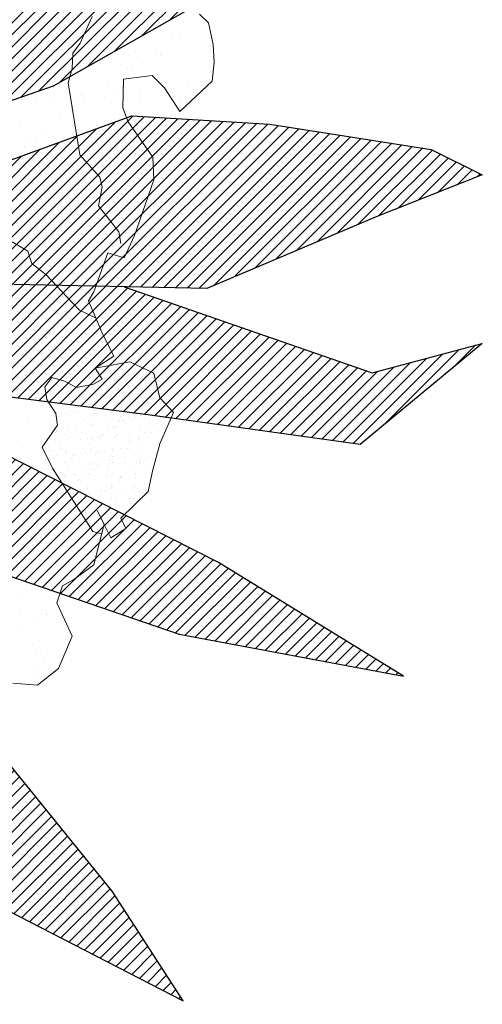
# Model space of a CAD drawing. Units: inches. Extents: x 1986 to 21484, y -1816 to 2016.
# Tile 71 of 85: x 3679.11 to 3687.55, y 1870.8 to 1888.79. Entities that reach past the tile are written whole.
import ezdxf

# ---------------------------------------------------------------- set-up
doc = ezdxf.new("R2010")
doc.units = ezdxf.units.IN
doc.layers.add('L-PLNT', color=84, linetype='Continuous', lineweight=13)
doc.layers.add('vfolhas', color=114, linetype='Continuous', lineweight=5)
for name, color, linetype in [('vfolha', 72, 'Continuous'), ('vfolha2', 110, 'Continuous'), ('vfolhas2', 102, 'Continuous')]:
    doc.layers.add(name, color=color, linetype=linetype)
pattern_1 = [(45, (-2446.5133113, 50.986076), (-0.004419417382, 0.004419417382), [])]

# ---------------------------------------------------------------- blocks, each defined once
blk = doc.blocks.new('arbusto_PB_verde_grande')
at = {"layer": 'vfolha2'}
h = blk.add_hatch(dxfattribs=at)
h.set_pattern_fill('ANSI31', color=256, scale=0.05, style=0)
h.set_pattern_definition(pattern_1)
h.paths.add_polyline_path([(0.02944, 0.35651), (0.00028, 0.09048), (0.02625, -0.03934), (0.047, 0.06233), (0.06189, 0.09731), (0.09372, 0.26573), (0.09955, 0.43473), (0.08789, 0.61313), (0.0645, 0.72266), (0.04988, 0.6851), (0.0236, 0.51294)])
h.paths.add_polyline_path([(0.30106, 0.43789), (0.14225, 0.24871), (0.26685, 0.30022)])
h.paths.add_polyline_path([(0.37995, 0.22817), (0.23697, 0.15193), (0.18428, 0.09364), (0.11122, 0.04358), (0.02625, -0.03934), (0.28061, 0.04667), (0.36829, 0.07798), (0.46756, 0.11239), (0.61068, 0.19376), (0.71585, 0.27823), (0.55813, 0.25948)])
h.paths.add_polyline_path([(0.56101, -0.29441), (0.72752, -0.32573), (0.59024, -0.2412), (0.42962, -0.15982), (0.02625, -0.03934), (0.14922, -0.14107), (0.18838, -0.16604), (0.41501, -0.24435)])
h.paths.add_polyline_path([(-0.27429, -0.44776), (-0.30352, -0.72628), (-0.23923, -0.64175), (-0.15457, -0.45716), (0.02625, -0.03934), (-0.16328, -0.25376)])
h.paths.add_polyline_path([(-0.51963, -0.24744), (-0.67736, -0.32573), (-0.59558, -0.35072), (-0.40574, -0.32882), (-0.21007, -0.20995), (0.02625, -0.03934), (-0.14874, -0.06595), (-0.31518, -0.09101), (-0.41452, -0.15048)])
h.paths.add_polyline_path([(-0.52546, 0.25007), (-0.70947, 0.24698), (-0.51963, 0.1093), (-0.32979, 0.02167), (-0.07567, -0.0128), (-0.04234, -0.02148), (-0.35024, 0.1312)])
at = {"layer": 'vfolhas'}
h = blk.add_hatch(dxfattribs=at)
h.set_pattern_fill('ANSI31', color=256, scale=0.05, style=0)
h.set_pattern_definition(pattern_1)
h.paths.add_polyline_path([(-0.07279, 0.50669), (-0.18085, 0.65063), (-0.2334, 0.67253), (-0.20712, 0.53176), (-0.10785, 0.25007), (0.02625, -0.03934), (0.00028, 0.09048), (0.00816, 0.16241), (-0.04939, 0.29079)])
h.paths.add_polyline_path([(0.09902, 0.41929), (0.09372, 0.26573), (0.07906, 0.18814), (0.15506, 0.36901), (0.26606, 0.5505), (0.28356, 0.63504), (0.2485, 0.68819), (0.25145, 0.63504), (0.20178, 0.54426)])
h.paths.add_polyline_path([(0.12295, 0.24073), (0.047, 0.06233), (0.02625, -0.03934), (0.11122, 0.04358), (0.18428, 0.09364), (0.27478, 0.19376), (0.3215, 0.25323), (0.44129, 0.38467), (0.47634, 0.57866), (0.41789, 0.45347), (0.28939, 0.30954)])
h.paths.add_polyline_path([(0.58145, -0.03779), (0.70707, 0.01536), (0.78591, 0.04667), (0.74796, 0.06549), (0.62818, 0.08423), (0.52595, 0.09048), (0.39745, 0.04358), (0.02625, -0.03934), (0.25728, -0.03154), (0.43834, -0.0347)])
h.paths.add_polyline_path([(0.52022, -0.03647), (0.43834, -0.0347), (0.25728, -0.03154), (0.02625, -0.03934), (0.17964, -0.08515), (0.53768, -0.13167), (0.69541, -0.15357), (0.78591, -0.07852), (0.70413, -0.10042)])
h.paths.add_polyline_path([(0.27189, -0.21929), (0.14922, -0.14107), (0.02625, -0.03934), (0.15794, -0.31007), (0.29522, -0.42585), (0.41789, -0.49157), (0.56396, -0.56669), (0.5114, -0.48532), (0.39456, -0.34139)])
h.paths.add_polyline_path([(-0.05818, -0.47591), (-0.02312, -0.61984), (0.047, -0.80134), (0.08494, -0.59794), (0.07911, -0.4071), (0.03527, -0.25376), (0.02625, -0.03934), (-0.03773, -0.26001)])
h.paths.add_polyline_path([(-0.24218, 0.14054), (-0.11073, 0.06858), (0.02625, -0.03934), (-0.04235, 0.10871), (-0.21007, 0.23757), (-0.36485, 0.33145), (-0.47874, 0.40341), (-0.54303, 0.46288), (-0.49041, 0.33145), (-0.39408, 0.22192)])
at = {"layer": 'vfolha'}
for p, q in [((0.52022, -0.03647), (0.70413, -0.10042)), ((0.78591, -0.07852), (0.69541, -0.15357)), ((0.70413, -0.10042), (0.78591, -0.07852)), ((0.53768, -0.13167), (0.17964, -0.08515)), ((0.69541, -0.15357), (0.53768, -0.13167)), ((0.5114, -0.48532), (0.39456, -0.34139)), ((0.56396, -0.56669), (0.5114, -0.48532)), ((0.41789, -0.49157), (0.56396, -0.56669))]:
    blk.add_line(p, q, dxfattribs=at)
at = {"layer": 'vfolha2'}
for p, q in [((0.61068, 0.19376), (0.46756, 0.11239)), ((0.59024, -0.2412), (0.42962, -0.15982)), ((0.72752, -0.32573), (0.59024, -0.2412)), ((0.41501, -0.24435), (0.56101, -0.29441)), ((0.56101, -0.29441), (0.72752, -0.32573))]:
    blk.add_line(p, q, dxfattribs=at)
at = {"layer": 'vfolhas2'}
for p, q in [((0.46756, 0.11239), (0.36829, 0.07798)), ((0.39745, 0.04358), (0.52595, 0.09048)), ((0.52595, 0.09048), (0.62818, 0.08423)), ((0.62818, 0.08423), (0.74796, 0.06549)), ((0.74796, 0.06549), (0.78591, 0.04667)), ((0.78591, 0.04667), (0.70707, 0.01536)), ((0.70707, 0.01536), (0.58145, -0.03779)), ((0.58145, -0.03779), (0.43834, -0.0347))]:
    blk.add_line(p, q, dxfattribs=at)
blk = doc.blocks.new('PLANT-SHRUB')
for p, q in [((2160.298, 1902.236), (2160.882, 1902.496)), ((2160.882, 1902.496), (2161.373, 1902.455)), ((2161.373, 1902.455), (2161.676, 1902.121)), ((2160.089, 1901.6), (2160.298, 1902.236)), ((2160.978, 1902.218), (2160.978, 1902.218)), ((2161.178, 1902.255), (2161.178, 1902.255)), ((2161.252, 1902.322), (2161.252, 1902.322)), ((2160.81, 1902.111), (2160.81, 1902.111)), ((2160.78, 1901.89), (2160.78, 1901.89)), ((2160.942, 1901.982), (2160.942, 1901.982)), ((2159.805, 1901.685), (2159.805, 1901.685)), ((2158.177, 1901.273), (2158.24, 1901.471)), ((2158.24, 1901.471), (2158.553, 1901.409)), ((2158.474, 1901.143), (2159.119, 1901.558)), ((2159.119, 1901.558), (2159.568, 1901.506)), ((2159.119, 1901.558), (2159.119, 1901.558)), ((2159.568, 1901.506), (2159.797, 1901.443)), ((2159.797, 1901.443), (2160.089, 1901.6)), ((2160.018, 1901.606), (2160.018, 1901.606)), ((2160.348, 1901.614), (2160.348, 1901.614)), ((2160.359, 1901.504), (2160.359, 1901.504)), ((2160.377, 1901.625), (2160.377, 1901.625)), ((2160.433, 1901.571), (2160.433, 1901.571)), ((2160.556, 1901.586), (2160.556, 1901.586)), ((2160.881, 1901.543), (2160.881, 1901.543)), ((2157.478, 1901.263), (2158.177, 1901.273)), ((2158.553, 1901.409), (2158.396, 1900.877)), ((2158.497, 1901.332), (2158.497, 1901.332)), ((2157.165, 1901.044), (2157.478, 1901.263)), ((2157.596, 1901.148), (2157.596, 1901.148)), ((2157.679, 1901.137), (2157.679, 1901.137)), ((2157.753, 1901.169), (2157.753, 1901.169)), ((2157.795, 1901.116), (2157.795, 1901.116)), ((2157.809, 1901.12), (2157.809, 1901.12)), ((2157.862, 1901.187), (2157.862, 1901.187)), ((2157.862, 1901.159), (2157.862, 1901.159)), ((2157.998, 1901.115), (2157.998, 1901.115)), ((2158.026, 1901.091), (2158.026, 1901.091)), ((2158.166, 1901.222), (2158.166, 1901.222)), ((2158.293, 1901.115), (2158.293, 1901.115)), ((2158.294, 1901.171), (2158.294, 1901.171)), ((2158.338, 1901.104), (2158.338, 1901.104)), ((2158.36, 1901.158), (2158.36, 1901.158)), ((2158.393, 1901.174), (2158.393, 1901.174)), ((2158.396, 1900.877), (2158.474, 1901.143)), ((2158.412, 1901.172), (2158.412, 1901.172)), ((2158.423, 1901.201), (2158.423, 1901.201)), ((2158.46, 1899.75), (2158.716, 1901.103)), ((2158.716, 1901.103), (2158.627, 1901.241)), ((2158.791, 1901.264), (2158.791, 1901.264)), ((2159.242, 1901.112), (2159.242, 1901.112)), ((2159.411, 1901.22), (2159.411, 1901.22)), ((2159.87, 1901.225), (2159.87, 1901.225)), ((2159.961, 1901.139), (2159.961, 1901.139)), ((2160.487, 1901.11), (2160.487, 1901.11)), ((2160.655, 1901.218), (2160.655, 1901.218)), ((2156.726, 1900.772), (2157.165, 1901.044)), ((2156.98, 1900.915), (2156.98, 1900.915)), ((2157.285, 1900.982), (2157.285, 1900.982)), ((2157.478, 1900.914), (2157.478, 1900.914)), ((2157.585, 1901.014), (2157.585, 1901.014)), ((2157.614, 1901.041), (2157.614, 1901.041)), ((2157.659, 1901.027), (2157.659, 1901.027)), ((2157.828, 1900.91), (2157.828, 1900.91)), ((2157.976, 1900.913), (2157.976, 1900.913)), ((2158.078, 1901.022), (2158.078, 1901.022)), ((2158.11, 1901.08), (2158.11, 1901.08)), ((2158.234, 1901.028), (2158.234, 1901.028)), ((2158.24, 1901.063), (2158.24, 1901.063)), ((2158.457, 1901.035), (2158.457, 1901.035)), ((2158.474, 1900.912), (2158.474, 1900.912)), ((2158.487, 1901.024), (2158.487, 1901.024)), ((2158.54, 1901.024), (2158.54, 1901.024)), ((2158.67, 1901.007), (2158.67, 1901.007)), ((2156.152, 1900.522), (2156.726, 1900.772)), ((2156.737, 1900.76), (2156.737, 1900.76)), ((2156.808, 1900.732), (2156.808, 1900.732)), ((2157.018, 1900.81), (2157.018, 1900.81)), ((2157.025, 1900.882), (2157.025, 1900.882)), ((2157.102, 1900.799), (2157.102, 1900.799)), ((2157.204, 1900.902), (2157.204, 1900.902)), ((2157.217, 1900.734), (2157.217, 1900.734)), ((2157.231, 1900.782), (2157.231, 1900.782)), ((2157.235, 1900.759), (2157.235, 1900.759)), ((2157.287, 1900.741), (2157.287, 1900.741)), ((2157.426, 1900.868), (2157.426, 1900.868)), ((2157.443, 1900.877), (2157.443, 1900.877)), ((2157.449, 1900.753), (2157.449, 1900.753)), ((2157.532, 1900.742), (2157.532, 1900.742)), ((2157.733, 1900.758), (2157.733, 1900.758)), ((2157.852, 1900.879), (2157.852, 1900.879)), ((2157.941, 1900.74), (2157.941, 1900.74)), ((2158.036, 1900.883), (2158.036, 1900.883)), ((2158.065, 1900.874), (2158.065, 1900.874)), ((2158.095, 1900.901), (2158.095, 1900.901)), ((2158.231, 1900.757), (2158.231, 1900.757)), ((2158.284, 1900.863), (2158.284, 1900.863)), ((2158.284, 1900.863), (2158.284, 1900.863)), ((2158.361, 1900.84), (2158.361, 1900.84)), ((2158.546, 1900.734), (2158.546, 1900.734)), ((2158.575, 1900.761), (2158.575, 1900.761)), ((2158.904, 1900.769), (2158.904, 1900.769)), ((2159.112, 1900.741), (2159.112, 1900.741)), ((2159.33, 1900.85), (2159.33, 1900.85)), ((2159.54, 1900.753), (2159.54, 1900.753)), ((2159.614, 1900.821), (2159.614, 1900.821)), ((2156.449, 1900.554), (2156.449, 1900.554)), ((2156.478, 1900.581), (2156.478, 1900.581)), ((2156.583, 1900.59), (2156.583, 1900.59)), ((2156.617, 1900.709), (2156.617, 1900.709)), ((2156.67, 1900.717), (2156.67, 1900.717)), ((2157.014, 1900.574), (2157.014, 1900.574)), ((2157.098, 1900.568), (2157.098, 1900.568)), ((2157.168, 1900.716), (2157.168, 1900.716)), ((2157.206, 1900.61), (2157.206, 1900.61)), ((2157.257, 1900.714), (2157.257, 1900.714)), ((2157.433, 1900.569), (2157.433, 1900.569)), ((2157.649, 1900.719), (2157.649, 1900.719)), ((2157.662, 1900.725), (2157.662, 1900.725)), ((2157.666, 1900.715), (2157.666, 1900.715)), ((2157.738, 1900.574), (2157.738, 1900.574)), ((2157.767, 1900.601), (2157.767, 1900.601)), ((2157.842, 1900.571), (2157.842, 1900.571)), ((2157.879, 1900.697), (2157.879, 1900.697)), ((2157.906, 1900.728), (2157.906, 1900.728)), ((2157.962, 1900.686), (2157.962, 1900.686)), ((2158.068, 1900.714), (2158.068, 1900.714)), ((2158.092, 1900.669), (2158.092, 1900.669)), ((2158.163, 1900.714), (2158.163, 1900.714)), ((2158.274, 1900.555), (2158.274, 1900.555)), ((2158.309, 1900.64), (2158.309, 1900.64)), ((2158.387, 1900.588), (2158.387, 1900.588)), ((2158.392, 1900.629), (2158.392, 1900.629)), ((2158.45, 1900.608), (2158.45, 1900.608)), ((2158.477, 1900.715), (2158.477, 1900.715)), ((2158.522, 1900.612), (2158.522, 1900.612)), ((2159.437, 1900.699), (2159.437, 1900.699)), ((2159.695, 1900.606), (2159.695, 1900.606)), ((2159.979, 1900.627), (2159.979, 1900.627)), ((2156.152, 1900.157), (2156.152, 1900.522)), ((2156.38, 1900.43), (2156.38, 1900.43)), ((2156.441, 1900.472), (2156.441, 1900.472)), ((2156.524, 1900.461), (2156.524, 1900.461)), ((2156.654, 1900.444), (2156.654, 1900.444)), ((2156.697, 1900.502), (2156.697, 1900.502)), ((2156.798, 1900.424), (2156.798, 1900.424)), ((2156.851, 1900.514), (2156.851, 1900.514)), ((2156.871, 1900.416), (2156.871, 1900.416)), ((2156.929, 1900.414), (2156.929, 1900.414)), ((2156.954, 1900.405), (2156.954, 1900.405)), ((2156.959, 1900.441), (2156.959, 1900.441)), ((2157.084, 1900.388), (2157.084, 1900.388)), ((2157.207, 1900.426), (2157.207, 1900.426)), ((2157.349, 1900.513), (2157.349, 1900.513)), ((2157.579, 1900.428), (2157.579, 1900.428)), ((2157.593, 1900.421), (2157.593, 1900.421)), ((2157.639, 1900.411), (2157.639, 1900.411)), ((2157.743, 1900.489), (2157.743, 1900.489)), ((2157.847, 1900.513), (2157.847, 1900.513)), ((2158.057, 1900.405), (2158.057, 1900.405)), ((2158.218, 1900.433), (2158.218, 1900.433)), ((2158.248, 1900.46), (2158.248, 1900.46)), ((2158.344, 1900.512), (2158.344, 1900.512)), ((2158.466, 1900.407), (2158.466, 1900.407)), ((2158.766, 1900.494), (2158.766, 1900.494)), ((2159.142, 1900.389), (2159.142, 1900.389)), ((2159.845, 1900.455), (2159.845, 1900.455)), ((2156.541, 1900.317), (2156.541, 1900.317)), ((2156.573, 1900.282), (2156.573, 1900.282)), ((2156.599, 1900.224), (2156.599, 1900.224)), ((2156.608, 1900.36), (2156.608, 1900.36)), ((2156.77, 1900.268), (2156.77, 1900.268)), ((2157.004, 1900.266), (2157.004, 1900.266)), ((2157.039, 1900.316), (2157.039, 1900.316)), ((2157.106, 1900.359), (2157.106, 1900.359)), ((2157.301, 1900.359), (2157.301, 1900.359)), ((2157.384, 1900.348), (2157.384, 1900.348)), ((2157.41, 1900.273), (2157.41, 1900.273)), ((2157.423, 1900.261), (2157.423, 1900.261)), ((2157.44, 1900.3), (2157.44, 1900.3)), ((2157.514, 1900.331), (2157.514, 1900.331)), ((2157.519, 1900.353), (2157.519, 1900.353)), ((2157.537, 1900.315), (2157.537, 1900.315)), ((2157.604, 1900.358), (2157.604, 1900.358)), ((2157.732, 1900.302), (2157.732, 1900.302)), ((2157.815, 1900.291), (2157.815, 1900.291)), ((2157.832, 1900.263), (2157.832, 1900.263)), ((2157.843, 1900.221), (2157.843, 1900.221)), ((2157.945, 1900.274), (2157.945, 1900.274)), ((2158.034, 1900.314), (2158.034, 1900.314)), ((2158.059, 1900.288), (2158.059, 1900.288)), ((2158.102, 1900.357), (2158.102, 1900.357)), ((2158.162, 1900.246), (2158.162, 1900.246)), ((2158.245, 1900.235), (2158.245, 1900.235)), ((2158.264, 1900.247), (2158.264, 1900.247)), ((2158.375, 1900.218), (2158.375, 1900.218)), ((2158.532, 1900.313), (2158.532, 1900.313)), ((2159.088, 1900.219), (2159.088, 1900.219)), ((2155.923, 1899.751), (2156.152, 1900.157)), ((2156.157, 1900.127), (2156.157, 1900.127)), ((2156.224, 1900.115), (2156.224, 1900.115)), ((2156.293, 1900.078), (2156.293, 1900.078)), ((2156.37, 1900.122), (2156.37, 1900.122)), ((2156.376, 1900.067), (2156.376, 1900.067)), ((2156.384, 1900.066), (2156.384, 1900.066)), ((2156.43, 1900.116), (2156.43, 1900.116)), ((2156.506, 1900.05), (2156.506, 1900.05)), ((2156.592, 1900.038), (2156.592, 1900.038)), ((2156.602, 1900.114), (2156.602, 1900.114)), ((2156.631, 1900.141), (2156.631, 1900.141)), ((2156.722, 1900.114), (2156.722, 1900.114)), ((2156.723, 1900.021), (2156.723, 1900.021)), ((2156.788, 1900.116), (2156.788, 1900.116)), ((2156.807, 1900.01), (2156.807, 1900.01)), ((2157.179, 1900.132), (2157.179, 1900.132)), ((2157.197, 1900.118), (2157.197, 1900.118)), ((2157.22, 1900.113), (2157.22, 1900.113)), ((2157.251, 1900.128), (2157.251, 1900.128)), ((2157.629, 1900.103), (2157.629, 1900.103)), ((2157.675, 1900.114), (2157.675, 1900.114)), ((2157.718, 1900.112), (2157.718, 1900.112)), ((2157.891, 1900.133), (2157.891, 1900.133)), ((2157.92, 1900.16), (2157.92, 1900.16)), ((2158.047, 1900.097), (2158.047, 1900.097)), ((2158.215, 1900.111), (2158.215, 1900.111)), ((2158.259, 1900.093), (2158.259, 1900.093)), ((2158.401, 1900.02), (2158.401, 1900.02)), ((2158.456, 1900.099), (2158.456, 1900.099)), ((2158.794, 1900.07), (2158.794, 1900.07)), ((2158.919, 1900.112), (2158.919, 1900.112)), ((2159.305, 1900.08), (2159.305, 1900.08)), ((2156.154, 1899.972), (2156.154, 1899.972)), ((2156.304, 1899.84), (2156.304, 1899.84)), ((2156.412, 1899.916), (2156.412, 1899.916)), ((2156.443, 1899.968), (2156.443, 1899.968)), ((2156.479, 1899.959), (2156.479, 1899.959)), ((2156.563, 1899.974), (2156.563, 1899.974)), ((2156.91, 1899.916), (2156.91, 1899.916)), ((2156.916, 1899.996), (2156.916, 1899.996)), ((2156.937, 1899.993), (2156.937, 1899.993)), ((2156.977, 1899.958), (2156.977, 1899.958)), ((2156.994, 1899.958), (2156.994, 1899.958)), ((2157.082, 1899.973), (2157.082, 1899.973)), ((2157.112, 1900), (2157.112, 1900)), ((2157.121, 1899.989), (2157.121, 1899.989)), ((2157.154, 1899.964), (2157.154, 1899.964)), ((2157.237, 1899.953), (2157.237, 1899.953)), ((2157.367, 1899.936), (2157.367, 1899.936)), ((2157.407, 1899.915), (2157.407, 1899.915)), ((2157.413, 1899.953), (2157.413, 1899.953)), ((2157.459, 1899.924), (2157.459, 1899.924)), ((2157.475, 1899.958), (2157.475, 1899.958)), ((2157.563, 1899.833), (2157.563, 1899.833)), ((2157.584, 1899.908), (2157.584, 1899.908)), ((2157.592, 1899.86), (2157.592, 1899.86)), ((2157.667, 1899.897), (2157.667, 1899.897)), ((2157.667, 1899.897), (2157.667, 1899.897)), ((2157.732, 1899.987), (2157.732, 1899.987)), ((2157.797, 1899.88), (2157.797, 1899.88)), ((2157.822, 1899.955), (2157.822, 1899.955)), ((2157.905, 1899.914), (2157.905, 1899.914)), ((2157.973, 1899.957), (2157.973, 1899.957)), ((2157.992, 1899.854), (2157.992, 1899.854)), ((2158.014, 1899.851), (2158.014, 1899.851)), ((2158.098, 1899.84), (2158.098, 1899.84)), ((2158.212, 1899.847), (2158.212, 1899.847)), ((2158.254, 1899.939), (2158.254, 1899.939)), ((2158.371, 1899.993), (2158.371, 1899.993)), ((2158.403, 1899.913), (2158.403, 1899.913)), ((2158.471, 1899.956), (2158.471, 1899.956)), ((2158.721, 1900.003), (2158.721, 1900.003)), ((2156.102, 1899.305), (2155.923, 1899.751)), ((2156.095, 1899.715), (2156.095, 1899.715)), ((2156.115, 1899.667), (2156.115, 1899.667)), ((2156.143, 1899.664), (2156.143, 1899.664)), ((2156.146, 1899.683), (2156.146, 1899.683)), ((2156.229, 1899.672), (2156.229, 1899.672)), ((2156.274, 1899.813), (2156.274, 1899.813)), ((2156.359, 1899.655), (2156.359, 1899.655)), ((2156.36, 1899.814), (2156.36, 1899.814)), ((2156.552, 1899.666), (2156.552, 1899.666)), ((2156.593, 1899.714), (2156.593, 1899.714)), ((2156.672, 1899.732), (2156.672, 1899.732)), ((2156.755, 1899.673), (2156.755, 1899.673)), ((2156.774, 1899.67), (2156.774, 1899.67)), ((2156.778, 1899.808), (2156.778, 1899.808)), ((2156.784, 1899.7), (2156.784, 1899.7)), ((2156.923, 1899.827), (2156.923, 1899.827)), ((2157.091, 1899.713), (2157.091, 1899.713)), ((2157.187, 1899.81), (2157.187, 1899.81)), ((2157.404, 1899.687), (2157.404, 1899.687)), ((2157.588, 1899.712), (2157.588, 1899.712)), ((2157.619, 1899.795), (2157.619, 1899.795)), ((2157.718, 1899.719), (2157.718, 1899.719)), ((2158.037, 1899.789), (2158.037, 1899.789)), ((2158.044, 1899.693), (2158.044, 1899.693)), ((2158.073, 1899.72), (2158.073, 1899.72)), ((2158.086, 1899.711), (2158.086, 1899.711)), ((2158.228, 1899.823), (2158.228, 1899.823)), ((2158.332, 1899.345), (2158.46, 1899.75)), ((2158.445, 1899.794), (2158.445, 1899.794)), ((2158.446, 1899.791), (2158.446, 1899.791)), ((2158.535, 1899.783), (2158.535, 1899.783)), ((2158.741, 1899.723), (2158.741, 1899.723)), ((2158.743, 1899.755), (2158.743, 1899.755)), ((2159.068, 1899.712), (2159.068, 1899.712)), ((2156.283, 1899.516), (2156.283, 1899.516)), ((2156.35, 1899.559), (2156.35, 1899.559)), ((2156.35, 1899.506), (2156.35, 1899.506)), ((2156.576, 1899.627), (2156.576, 1899.627)), ((2156.596, 1899.527), (2156.596, 1899.527)), ((2156.659, 1899.616), (2156.659, 1899.616)), ((2156.7, 1899.603), (2156.7, 1899.603)), ((2156.768, 1899.5), (2156.768, 1899.5)), ((2156.78, 1899.515), (2156.78, 1899.515)), ((2156.789, 1899.598), (2156.789, 1899.598)), ((2156.848, 1899.558), (2156.848, 1899.558)), ((2156.883, 1899.609), (2156.883, 1899.609)), ((2156.984, 1899.65), (2156.984, 1899.65)), ((2157.006, 1899.57), (2157.006, 1899.57)), ((2157.09, 1899.559), (2157.09, 1899.559)), ((2157.177, 1899.502), (2157.177, 1899.502)), ((2157.22, 1899.542), (2157.22, 1899.542)), ((2157.235, 1899.533), (2157.235, 1899.533)), ((2157.265, 1899.56), (2157.265, 1899.56)), ((2157.278, 1899.514), (2157.278, 1899.514)), ((2157.346, 1899.557), (2157.346, 1899.557)), ((2157.403, 1899.645), (2157.403, 1899.645)), ((2157.437, 1899.513), (2157.437, 1899.513)), ((2157.52, 1899.502), (2157.52, 1899.502)), ((2157.609, 1899.487), (2157.609, 1899.487)), ((2157.65, 1899.485), (2157.65, 1899.485)), ((2157.776, 1899.513), (2157.776, 1899.513)), ((2157.812, 1899.647), (2157.812, 1899.647)), ((2157.844, 1899.556), (2157.844, 1899.556)), ((2157.884, 1899.547), (2157.884, 1899.547)), ((2158.027, 1899.481), (2158.027, 1899.481)), ((2158.127, 1899.607), (2158.127, 1899.607)), ((2158.243, 1899.631), (2158.243, 1899.631)), ((2158.274, 1899.512), (2158.274, 1899.512)), ((2158.323, 1899.638), (2158.323, 1899.638)), ((2158.341, 1899.555), (2158.341, 1899.555)), ((2156.162, 1899.266), (2156.102, 1899.305)), ((2156.427, 1899.373), (2156.427, 1899.373)), ((2156.457, 1899.4), (2156.457, 1899.4)), ((2156.464, 1899.313), (2156.464, 1899.313)), ((2156.542, 1899.358), (2156.542, 1899.358)), ((2156.961, 1899.312), (2156.961, 1899.312)), ((2156.974, 1899.342), (2156.974, 1899.342)), ((2157.076, 1899.387), (2157.076, 1899.387)), ((2157.154, 1899.362), (2157.154, 1899.362)), ((2157.393, 1899.337), (2157.393, 1899.337)), ((2157.459, 1899.312), (2157.459, 1899.312)), ((2157.716, 1899.392), (2157.716, 1899.392)), ((2157.745, 1899.419), (2157.745, 1899.419)), ((2157.802, 1899.339), (2157.802, 1899.339)), ((2157.859, 1899.242), (2158.332, 1899.345)), ((2157.867, 1899.457), (2157.867, 1899.457)), ((2157.95, 1899.446), (2157.95, 1899.446)), ((2157.957, 1899.311), (2157.957, 1899.311)), ((2157.975, 1899.32), (2157.975, 1899.32)), ((2158.08, 1899.429), (2158.08, 1899.429)), ((2158.233, 1899.323), (2158.233, 1899.323)), ((2158.297, 1899.4), (2158.297, 1899.4)), ((2158.332, 1899.345), (2158.332, 1899.345)), ((2156.642, 1898.953), (2156.162, 1899.266)), ((2156.302, 1899.238), (2156.302, 1899.238)), ((2156.34, 1899.198), (2156.34, 1899.198)), ((2156.429, 1899.232), (2156.429, 1899.232)), ((2156.512, 1899.221), (2156.512, 1899.221)), ((2156.642, 1899.204), (2156.642, 1899.204)), ((2156.642, 1898.953), (2156.685, 1899.186)), ((2156.651, 1899.115), (2156.651, 1899.115)), ((2156.685, 1899.186), (2156.865, 1899.149)), ((2156.758, 1899.192), (2156.758, 1899.192)), ((2156.859, 1899.175), (2156.859, 1899.175)), ((2156.865, 1899.149), (2157.131, 1898.976)), ((2156.908, 1899.232), (2156.908, 1899.232)), ((2156.937, 1899.259), (2156.937, 1899.259)), ((2156.942, 1899.164), (2156.942, 1899.164)), ((2157.072, 1899.147), (2157.072, 1899.147)), ((2157.149, 1899.114), (2157.149, 1899.114)), ((2157.167, 1899.194), (2157.167, 1899.194)), ((2157.217, 1899.157), (2157.217, 1899.157)), ((2157.289, 1899.119), (2157.289, 1899.119)), ((2157.352, 1899.113), (2157.352, 1899.113)), ((2157.418, 1899.119), (2157.418, 1899.119)), ((2157.521, 1899.22), (2157.521, 1899.22)), ((2157.557, 1899.247), (2157.557, 1899.247)), ((2157.599, 1899.179), (2157.599, 1899.179)), ((2157.647, 1899.113), (2157.647, 1899.113)), ((2157.714, 1899.156), (2157.714, 1899.156)), ((2157.732, 1899.068), (2157.859, 1899.242)), ((2157.902, 1899.252), (2157.902, 1899.252)), ((2158.597, 1899.111), (2158.597, 1899.111)), ((2158.765, 1899.218), (2158.765, 1899.218)), ((2156.12, 1898.599), (2156.245, 1899.026)), ((2156.245, 1899.026), (2156.642, 1898.953)), ((2156.647, 1898.962), (2156.647, 1898.962)), ((2157.091, 1898.938), (2157.091, 1898.938)), ((2157.131, 1898.976), (2157.212, 1898.745)), ((2157.229, 1898.946), (2157.229, 1898.946)), ((2157.373, 1899.108), (2157.373, 1899.108)), ((2157.383, 1899.029), (2157.383, 1899.029)), ((2157.388, 1899.092), (2157.388, 1899.092)), ((2157.503, 1899.091), (2157.503, 1899.091)), ((2157.674, 1898.768), (2157.732, 1899.068)), ((2157.693, 1898.948), (2157.693, 1898.948)), ((2157.72, 1899.062), (2157.72, 1899.062)), ((2157.299, 1898.911), (2157.299, 1898.911)), ((2157.33, 1898.911), (2157.33, 1898.911)), ((2157.504, 1898.888), (2157.504, 1898.888)), ((2157.547, 1898.572), (2157.674, 1898.768)), ((2157.585, 1898.756), (2157.585, 1898.756)), ((2157.589, 1898.871), (2157.589, 1898.871)), ((2157.624, 1898.868), (2157.624, 1898.868)), ((2158.167, 1898.796), (2158.167, 1898.796)), ((2155.89, 1897.973), (2156.12, 1898.599)), ((2156.56, 1898.608), (2156.56, 1898.608)), ((2157.129, 1898.592), (2157.129, 1898.592)), ((2157.212, 1898.745), (2157.339, 1898.537)), ((2157.339, 1898.537), (2157.547, 1898.572)), ((2157.355, 1898.696), (2157.355, 1898.696)), ((2157.372, 1898.721), (2157.372, 1898.721)), ((2157.518, 1898.713), (2157.518, 1898.713)), ((2157.541, 1898.652), (2157.541, 1898.652)), ((2157.571, 1898.679), (2157.571, 1898.679)), ((2157.572, 1898.668), (2157.572, 1898.668)), ((2157.805, 1898.606), (2157.805, 1898.606)), ((2157.082, 1898.501), (2157.082, 1898.501)), ((2157.156, 1898.569), (2157.156, 1898.569)), ((2156.127, 1897.984), (2156.005, 1898.286)), ((2157.198, 1898.22), (2157.198, 1898.22)), ((2156.622, 1898.192), (2156.622, 1898.192)), ((2156.685, 1898.137), (2156.685, 1898.137)), ((2157.029, 1898.112), (2157.029, 1898.112)), ((2157.668, 1898.178), (2157.668, 1898.178)), ((2155.032, 1897.574), (2155.703, 1897.921)), ((2155.703, 1897.921), (2155.89, 1897.973)), ((2156.127, 1897.799), (2156.127, 1897.984)), ((2156.179, 1898.023), (2156.179, 1898.023)), ((2156.722, 1897.952), (2156.722, 1897.952)), ((2156.93, 1897.924), (2156.93, 1897.924)), ((2157.255, 1897.881), (2157.255, 1897.881)), ((2153.508, 1897.178), (2154.458, 1897.678)), ((2154.458, 1897.678), (2154.876, 1897.845)), ((2154.876, 1897.845), (2155.032, 1897.574)), ((2156.081, 1897.817), (2156.081, 1897.817)), ((2156.127, 1897.097), (2156.127, 1897.799)), ((2156.263, 1897.751), (2156.263, 1897.751)), ((2156.337, 1897.818), (2156.337, 1897.818)), ((2157.104, 1897.822), (2157.104, 1897.822)), ((2154.623, 1897.434), (2154.74, 1897.616)), ((2154.74, 1897.616), (2154.74, 1897.616)), ((2156.237, 1897.608), (2156.237, 1897.608)), ((2154.243, 1897.351), (2154.243, 1897.351)), ((2154.316, 1897.418), (2154.316, 1897.418)), ((2154.495, 1897.456), (2154.495, 1897.456)), ((2154.597, 1897.146), (2154.623, 1897.434)), ((2155.865, 1897.386), (2155.865, 1897.386)), ((2156.596, 1897.422), (2156.596, 1897.422)), ((2153.237, 1896.865), (2153.508, 1897.178)), ((2154.202, 1897.249), (2154.202, 1897.249)), ((2154.386, 1897.223), (2154.386, 1897.223)), ((2154.41, 1897.221), (2154.41, 1897.221)), ((2154.571, 1896.833), (2154.597, 1897.146)), ((2154.735, 1897.178), (2154.735, 1897.178)), ((2155.63, 1897.221), (2155.63, 1897.221)), ((2156.875, 1897.219), (2156.875, 1897.219)), ((2153.845, 1896.986), (2153.845, 1896.986)), ((2153.93, 1897.099), (2153.93, 1897.099)), ((2154.217, 1897.116), (2154.217, 1897.116)), ((2155.01, 1897.06), (2155.01, 1897.06)), ((2155.278, 1897.107), (2155.278, 1897.107)), ((2155.444, 1897), (2155.444, 1897)), ((2155.462, 1897.114), (2155.462, 1897.114)), ((2155.486, 1897.08), (2155.486, 1897.08)), ((2155.518, 1897.068), (2155.518, 1897.068)), ((2155.811, 1897.037), (2155.811, 1897.037)), ((2156.056, 1897.047), (2156.056, 1897.047)), ((2156.127, 1897.097), (2156.127, 1897.097)), ((2156.179, 1896.769), (2156.127, 1897.097)), ((2156.354, 1896.965), (2156.354, 1896.965)), ((2156.707, 1897.111), (2156.707, 1897.111)), ((2153.122, 1896.083), (2153.237, 1896.865)), ((2153.237, 1896.865), (2153.237, 1896.865)), ((2154.283, 1896.624), (2154.571, 1896.833)), ((2156.562, 1896.938), (2156.562, 1896.938)), ((2151.233, 1896.364), (2151.494, 1896.594)), ((2151.494, 1896.594), (2152.308, 1896.594)), ((2152.308, 1896.594), (2152.214, 1896.083)), ((2153.423, 1896.699), (2153.423, 1896.699)), ((2153.423, 1896.6), (2153.423, 1896.6)), ((2153.425, 1896.611), (2153.425, 1896.611)), ((2153.497, 1896.668), (2153.497, 1896.668)), ((2154.192, 1896.467), (2154.283, 1896.624)), ((2154.469, 1896.686), (2154.469, 1896.686)), ((2154.67, 1896.609), (2154.67, 1896.609)), ((2155.046, 1896.636), (2155.046, 1896.636)), ((2155.492, 1896.69), (2155.492, 1896.69)), ((2155.914, 1896.607), (2155.914, 1896.607)), ((2156.076, 1896.553), (2156.179, 1896.769)), ((2151.89, 1896.518), (2151.89, 1896.518)), ((2152.215, 1896.475), (2152.215, 1896.475)), ((2154.178, 1895.919), (2154.192, 1896.467)), ((2156.169, 1896.234), (2156.076, 1896.553)), ((2151.025, 1896.114), (2151.233, 1896.364)), ((2151.837, 1896.337), (2151.837, 1896.337)), ((2152.966, 1896.377), (2152.966, 1896.377)), ((2153.026, 1896.236), (2153.026, 1896.236)), ((2153.291, 1896.334), (2153.291, 1896.334)), ((2153.834, 1896.262), (2153.834, 1896.262)), ((2153.905, 1896.329), (2153.905, 1896.329)), ((2154.042, 1896.235), (2154.042, 1896.235)), ((2154.625, 1896.249), (2154.625, 1896.249)), ((2154.698, 1896.317), (2154.698, 1896.317)), ((2154.985, 1896.29), (2154.985, 1896.29)), ((2150.816, 1895.77), (2151.025, 1896.114)), ((2152.214, 1896.083), (2152.225, 1895.77)), ((2153.018, 1895.833), (2153.122, 1896.083)), ((2153.894, 1896.115), (2153.894, 1896.115)), ((2154.063, 1896.223), (2154.063, 1896.223)), ((2154.367, 1896.192), (2154.367, 1896.192)), ((2154.91, 1896.121), (2154.91, 1896.121)), ((2155.118, 1896.093), (2155.118, 1896.093)), ((2155.139, 1896.113), (2155.139, 1896.113)), ((2155.308, 1896.22), (2155.308, 1896.22)), ((2152.319, 1895.968), (2152.319, 1895.968)), ((2152.678, 1895.917), (2152.678, 1895.917)), ((2153.398, 1895.929), (2153.398, 1895.929)), ((2153.432, 1894.817), (2154.178, 1895.919)), ((2154.178, 1895.919), (2154.178, 1895.919)), ((2154.227, 1895.885), (2154.227, 1895.885)), ((2154.444, 1895.915), (2154.444, 1895.915)), ((2155.442, 1896.05), (2155.442, 1896.05)), ((2155.467, 1895.92), (2155.467, 1895.92)), ((2150.827, 1895.541), (2150.816, 1895.77)), ((2152.225, 1895.77), (2152.653, 1895.457)), ((2152.604, 1895.85), (2152.604, 1895.85)), ((2152.653, 1895.457), (2153.018, 1895.833)), ((2151.314, 1895.559), (2151.314, 1895.559)), ((2151.522, 1895.532), (2151.522, 1895.532)), ((2151.811, 1895.567), (2151.811, 1895.567)), ((2151.858, 1895.613), (2151.858, 1895.613)), ((2152.858, 1895.554), (2152.858, 1895.554)), ((2153.102, 1895.61), (2153.102, 1895.61)), ((2153.879, 1895.566), (2153.879, 1895.566)), ((2153.88, 1895.559), (2153.88, 1895.559)), ((2154.347, 1895.608), (2154.347, 1895.608)), ((2154.959, 1895.52), (2154.959, 1895.52)), ((2151.847, 1895.489), (2151.847, 1895.489)), ((2152.206, 1895.485), (2152.206, 1895.485)), ((2152.389, 1895.418), (2152.389, 1895.418)), ((2152.597, 1895.39), (2152.597, 1895.39)), ((2152.653, 1895.457), (2152.653, 1895.457)), ((2152.922, 1895.347), (2152.922, 1895.347)), ((2153.806, 1895.499), (2153.806, 1895.499)), ((2151.859, 1895.166), (2151.859, 1895.166)), ((2152.293, 1895.198), (2152.293, 1895.198)), ((2152.496, 1895.224), (2152.496, 1895.224)), ((2153.373, 1895.159), (2153.373, 1895.159)), ((2153.465, 1895.276), (2153.465, 1895.276)), ((2153.673, 1895.249), (2153.673, 1895.249)), ((2153.74, 1895.222), (2153.74, 1895.222)), ((2153.998, 1895.206), (2153.998, 1895.206)), ((2154.985, 1895.219), (2154.985, 1895.219)), ((2151.785, 1895.099), (2151.785, 1895.099)), ((2152.327, 1895.117), (2152.327, 1895.117)), ((2153.408, 1895.134), (2153.408, 1895.134)), ((2153.572, 1895.114), (2153.572, 1895.114)), ((2154.419, 1895.145), (2154.419, 1895.145)), ((2154.541, 1895.134), (2154.541, 1895.134)), ((2154.749, 1895.107), (2154.749, 1895.107)), ((2154.816, 1895.112), (2154.816, 1895.112)), ((2151.786, 1894.797), (2151.786, 1894.797)), ((2153.06, 1894.816), (2153.06, 1894.816)), ((2153.197, 1894.674), (2153.432, 1894.817)), ((2153.432, 1894.817), (2153.432, 1894.817)), ((2152.832, 1894.784), (2152.832, 1894.784)), ((2152.986, 1894.748), (2152.986, 1894.748)), ((2153.001, 1894.478), (2153.197, 1894.674)), ((2153.855, 1894.789), (2153.855, 1894.789)), ((2154.609, 1894.784), (2154.609, 1894.784)), ((2152.282, 1894.23), (2152.778, 1894.439)), ((2152.778, 1894.439), (2153.001, 1894.478)), ((2152.78, 1894.61), (2152.78, 1894.61)), ((2154.024, 1894.607), (2154.024, 1894.607)), ((2154.262, 1894.465), (2154.262, 1894.465)), ((2152.229, 1894.404), (2152.229, 1894.404)), ((2152.268, 1894.427), (2152.268, 1894.427)), ((2152.554, 1894.361), (2152.554, 1894.361)), ((2152.589, 1894.384), (2152.589, 1894.384)), ((2153.097, 1894.29), (2153.097, 1894.29)), ((2153.305, 1894.262), (2153.305, 1894.262)), ((2153.348, 1894.389), (2153.348, 1894.389)), ((2154.188, 1894.397), (2154.188, 1894.397)), ((2153.249, 1894.113), (2153.249, 1894.113)), ((2153.417, 1894.221), (2153.417, 1894.221)), ((2153.63, 1894.22), (2153.63, 1894.22)), ((2152.807, 1894.014), (2152.807, 1894.014)), ((2153.79, 1894.033), (2153.79, 1894.033)), ((2153.83, 1894.019), (2153.83, 1894.019)), ((2153.442, 1893.714), (2153.442, 1893.714)), ((2153.322, 1893.618), (2153.322, 1893.618)), ((2153.369, 1893.647), (2153.369, 1893.647))]:
    blk.add_line(p, q)

msp = doc.modelspace()

# ---------------------------------------------------------------- block references
at = {"layer": 'L-PLNT', "rotation": 223.1883365522388}
msp.add_blockref('PLANT-SHRUB', (3953.27, 4742.965), dxfattribs=at)
at = {"layer": 'L-PLNT', "xscale": 24.60366729364114, "yscale": 24.60366729364114, "zscale": 24.60366729364114}
msp.add_blockref('arbusto_PB_verde_grande', (3668.218, 1884.805), dxfattribs=at)

doc.saveas('drawing.dxf')
